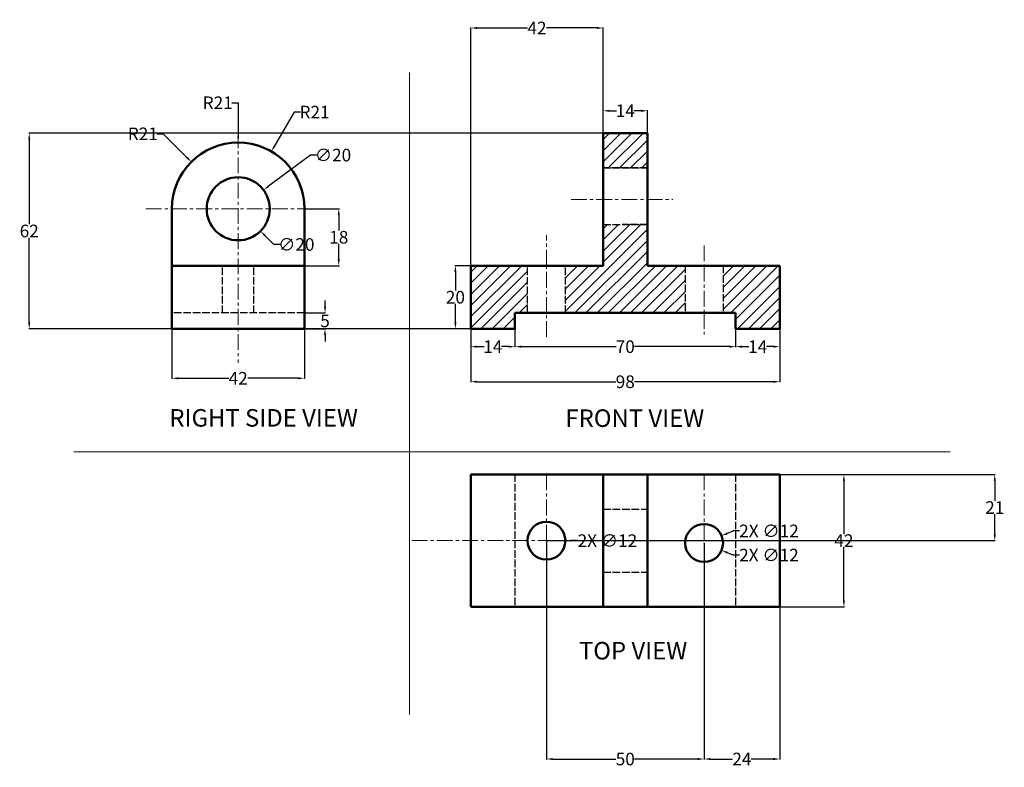
# Model space of a CAD drawing. Units: millimetres. Extents: x -145 to 168, y -286 to 127.
# Tile 1 of 2: x -145 to 168, y -286 to -49. Entities that reach past the tile are written whole.
import ezdxf

# ---------------------------------------------------------------- set-up
doc = ezdxf.new("R2010")
doc.units = ezdxf.units.MM
doc.header["$MEASUREMENT"] = 0
doc.linetypes.add('ACAD_ISO02W100', pattern=[15, 12, -3])
doc.linetypes.add('CENTER', pattern=[2, 1.25, -0.25, 0.25, -0.25])
for name, color, linetype, lineweight in [('M-CNTR', 1, 'CENTER', 18), ('M-CONS', 8, 'Continuous', 18), ('M-DIMS', 2, 'Continuous', 25), ('M-HATC', 8, 'Continuous', 18), ('M-HIDN', 6, 'ACAD_ISO02W100', 25), ('M-OUTL', 7, 'Continuous', 50), ('M-TEXT', 3, 'Continuous', 25)]:
    doc.layers.add(name, color=color, linetype=linetype, lineweight=lineweight)
doc.styles.get("Standard").update_dxf_attribs({"font": 'arial.ttf'})
doc.dimstyles.get("Standard").update_dxf_attribs({"dimtxt": 4, "dimasz": 2, "dimexe": 0.18, "dimexo": 0.0625, "dimgap": 0.09, "dimtad": 0, "dimtih": 1, "dimtoh": 1, "dimdec": 0, "dimzin": 0, "dimdsep": 46, "dimtxsty": 'Standard', "dimcen": 0.09, "dimadec": 0, "dimazin": 0, "dimtfac": 1, "dimtdec": 0, "dimtofl": 0, "dimtmove": 0, "dimatfit": 3, "dimfxl": 1, "dimtolj": 1, "dimtzin": 0, "dimarcsym": 0})

# ---------------------------------------------------------------- blocks, each defined once
blk = doc.blocks.new('*D12')
at = {"layer": 'Defpoints', "color": 0, "transparency": 16777216}
for p in [(40.45, -78.33), (40.45, -85.43), (54.45, -85.43)]:
    blk.add_point(p, dxfattribs=at)
at = {"layer": 'M-DIMS', "color": 0, "lineweight": -2, "transparency": 16777216}
for p, q in [((40.45, -85.37), (40.45, -78.15)), ((42.45, -78.33), (44.69, -78.33)), ((52.45, -78.33), (50.21, -78.33)), ((54.45, -85.37), (54.45, -78.15))]:
    blk.add_line(p, q, dxfattribs=at)
at = {"layer": 'M-DIMS', "color": 0, "transparency": 16777216}
for points in [[(42.45, -78), (42.45, -78.67), (40.45, -78.33)], [(52.45, -78), (52.45, -78.67), (54.45, -78.33)]]:
    blk.add_solid(points, dxfattribs=at)
at = {"layer": 'M-DIMS', "color": 0, "transparency": 16777216, "insert": (47.45, -78.33), "char_height": 4, "attachment_point": 5}
blk.add_mtext('\\A1;14', dxfattribs=at)
blk = doc.blocks.new('*D13')
at = {"layer": 'Defpoints', "color": 0, "transparency": 16777216}
for p in [(-6.42, -127.43), (-1.55, -127.43), (-1.55, -147.43)]:
    blk.add_point(p, dxfattribs=at)
at = {"layer": 'M-DIMS', "color": 0, "lineweight": -2, "transparency": 16777216}
for p, q in [((-1.61, -127.43), (-6.6, -127.43)), ((-6.42, -129.43), (-6.42, -135.3)), ((-6.42, -145.43), (-6.42, -139.56)), ((-1.61, -147.43), (-6.6, -147.43))]:
    blk.add_line(p, q, dxfattribs=at)
at = {"layer": 'M-DIMS', "color": 0, "transparency": 16777216}
for points in [[(-6.75, -129.43), (-6.08, -129.43), (-6.42, -127.43)], [(-6.75, -145.43), (-6.08, -145.43), (-6.42, -147.43)]]:
    blk.add_solid(points, dxfattribs=at)
at = {"layer": 'M-DIMS', "color": 0, "transparency": 16777216, "insert": (-6.42, -137.43), "char_height": 4, "attachment_point": 5}
blk.add_mtext('\\A1;20', dxfattribs=at)
blk = doc.blocks.new('*D14')
at = {"layer": 'Defpoints', "color": 0, "transparency": 16777216}
for p in [(-1.55, -147.43), (12.45, -147.43), (12.45, -153.1)]:
    blk.add_point(p, dxfattribs=at)
at = {"layer": 'M-DIMS', "color": 0, "lineweight": -2, "transparency": 16777216}
for p, q in [((-1.55, -147.49), (-1.55, -153.28)), ((12.45, -147.49), (12.45, -153.28)), ((0.45, -153.1), (2.69, -153.1)), ((10.45, -153.1), (8.21, -153.1))]:
    blk.add_line(p, q, dxfattribs=at)
at = {"layer": 'M-DIMS', "color": 0, "transparency": 16777216}
for points in [[(0.45, -152.77), (0.45, -153.44), (-1.55, -153.1)], [(10.45, -152.77), (10.45, -153.44), (12.45, -153.1)]]:
    blk.add_solid(points, dxfattribs=at)
at = {"layer": 'M-DIMS', "color": 0, "transparency": 16777216, "insert": (5.45, -153.1), "char_height": 4, "attachment_point": 5}
blk.add_mtext('\\A1;14', dxfattribs=at)
blk = doc.blocks.new('*D15')
at = {"layer": 'Defpoints', "color": 0, "transparency": 16777216}
for p in [(12.45, -142.43), (82.45, -142.43), (82.45, -153.1)]:
    blk.add_point(p, dxfattribs=at)
at = {"layer": 'M-DIMS', "color": 0, "lineweight": -2, "transparency": 16777216}
for p, q in [((12.45, -142.49), (12.45, -153.28)), ((82.45, -142.49), (82.45, -153.28)), ((14.45, -153.1), (44.52, -153.1)), ((80.45, -153.1), (50.38, -153.1))]:
    blk.add_line(p, q, dxfattribs=at)
at = {"layer": 'M-DIMS', "color": 0, "transparency": 16777216}
for points in [[(14.45, -152.77), (14.45, -153.44), (12.45, -153.1)], [(80.45, -152.77), (80.45, -153.44), (82.45, -153.1)]]:
    blk.add_solid(points, dxfattribs=at)
at = {"layer": 'M-DIMS', "color": 0, "transparency": 16777216, "insert": (47.45, -153.1), "char_height": 4, "attachment_point": 5}
blk.add_mtext('\\A1;70', dxfattribs=at)
blk = doc.blocks.new('*D16')
at = {"layer": 'Defpoints', "color": 0, "transparency": 16777216}
for p in [(82.45, -147.43), (96.45, -147.43), (96.45, -153.1)]:
    blk.add_point(p, dxfattribs=at)
at = {"layer": 'M-DIMS', "color": 0, "lineweight": -2, "transparency": 16777216}
for p, q in [((82.45, -147.49), (82.45, -153.28)), ((96.45, -147.49), (96.45, -153.28)), ((84.45, -153.1), (86.69, -153.1)), ((94.45, -153.1), (92.21, -153.1))]:
    blk.add_line(p, q, dxfattribs=at)
at = {"layer": 'M-DIMS', "color": 0, "transparency": 16777216}
for points in [[(84.45, -152.77), (84.45, -153.44), (82.45, -153.1)], [(94.45, -152.77), (94.45, -153.44), (96.45, -153.1)]]:
    blk.add_solid(points, dxfattribs=at)
at = {"layer": 'M-DIMS', "color": 0, "transparency": 16777216, "insert": (89.45, -153.1), "char_height": 4, "attachment_point": 5}
blk.add_mtext('\\A1;14', dxfattribs=at)
blk = doc.blocks.new('*D17')
at = {"layer": 'Defpoints', "color": 0, "transparency": 16777216}
for p in [(96.45, -193.6), (116.79, -193.6), (96.45, -235.6)]:
    blk.add_point(p, dxfattribs=at)
at = {"layer": 'M-DIMS', "color": 0, "lineweight": -2, "transparency": 16777216}
for p, q in [((96.51, -193.6), (116.97, -193.6)), ((116.79, -195.6), (116.79, -212.5)), ((116.79, -233.6), (116.79, -216.7)), ((96.51, -235.6), (116.97, -235.6))]:
    blk.add_line(p, q, dxfattribs=at)
at = {"layer": 'M-DIMS', "color": 0, "transparency": 16777216}
for points in [[(116.46, -195.6), (117.13, -195.6), (116.79, -193.6)], [(116.46, -233.6), (117.13, -233.6), (116.79, -235.6)]]:
    blk.add_solid(points, dxfattribs=at)
at = {"layer": 'M-DIMS', "color": 0, "transparency": 16777216, "insert": (116.79, -214.6), "char_height": 4, "attachment_point": 5}
blk.add_mtext('\\A1;42', dxfattribs=at)
blk = doc.blocks.new('*D18')
at = {"layer": 'Defpoints', "color": 0, "transparency": 16777216}
for p in [(-1.55, -147.43), (96.45, -147.43), (96.45, -164.22)]:
    blk.add_point(p, dxfattribs=at)
at = {"layer": 'M-DIMS', "color": 0, "lineweight": -2, "transparency": 16777216}
for p, q in [((-1.55, -147.49), (-1.55, -164.4)), ((96.45, -147.49), (96.45, -164.4)), ((0.45, -164.22), (44.49, -164.22)), ((94.45, -164.22), (50.41, -164.22))]:
    blk.add_line(p, q, dxfattribs=at)
at = {"layer": 'M-DIMS', "color": 0, "transparency": 16777216}
for points in [[(0.45, -163.89), (0.45, -164.56), (-1.55, -164.22)], [(94.45, -163.89), (94.45, -164.56), (96.45, -164.22)]]:
    blk.add_solid(points, dxfattribs=at)
at = {"layer": 'M-DIMS', "color": 0, "transparency": 16777216, "insert": (47.45, -164.22), "char_height": 4, "attachment_point": 5}
blk.add_mtext('\\A1;98', dxfattribs=at)
blk = doc.blocks.new('*D19')
at = {"layer": 'Defpoints', "color": 0, "transparency": 16777216}
for p in [(-96.3, -147.43), (-54.3, -147.43), (-96.3, -163.13)]:
    blk.add_point(p, dxfattribs=at)
at = {"layer": 'M-DIMS', "color": 0, "lineweight": -2, "transparency": 16777216}
for p, q in [((-96.3, -147.49), (-96.3, -163.31)), ((-54.3, -147.49), (-54.3, -163.31)), ((-94.3, -163.13), (-78.31, -163.13)), ((-56.3, -163.13), (-72.28, -163.13))]:
    blk.add_line(p, q, dxfattribs=at)
at = {"layer": 'M-DIMS', "color": 0, "transparency": 16777216}
for points in [[(-94.3, -162.8), (-94.3, -163.46), (-96.3, -163.13)], [(-56.3, -162.8), (-56.3, -163.46), (-54.3, -163.13)]]:
    blk.add_solid(points, dxfattribs=at)
at = {"layer": 'M-DIMS', "color": 0, "transparency": 16777216, "insert": (-75.3, -163.13), "char_height": 4, "attachment_point": 5}
blk.add_mtext('\\A1;42', dxfattribs=at)
blk = doc.blocks.new('*D20')
at = {"layer": 'Defpoints', "color": 0, "transparency": 16777216}
for p in [(-54.3, -142.43), (-47.76, -142.43), (-54.3, -147.43)]:
    blk.add_point(p, dxfattribs=at)
at = {"layer": 'M-DIMS', "color": 0, "lineweight": -2, "transparency": 16777216}
for p, q in [((-47.76, -140.43), (-47.76, -138.43)), ((-54.24, -142.43), (-47.58, -142.43)), ((-54.24, -147.43), (-47.58, -147.43)), ((-47.76, -149.43), (-47.76, -151.43))]:
    blk.add_line(p, q, dxfattribs=at)
at = {"layer": 'M-DIMS', "color": 0, "transparency": 16777216}
for points in [[(-48.09, -140.43), (-47.43, -140.43), (-47.76, -142.43)], [(-48.09, -149.43), (-47.43, -149.43), (-47.76, -147.43)]]:
    blk.add_solid(points, dxfattribs=at)
at = {"layer": 'M-DIMS', "color": 0, "transparency": 16777216, "insert": (-47.76, -144.93), "char_height": 4, "attachment_point": 5}
blk.add_mtext('\\A1;5', dxfattribs=at)
blk = doc.blocks.new('*D21')
at = {"layer": 'Defpoints', "color": 0, "transparency": 16777216}
for p in [(-54.3, -109.39), (-54.3, -127.43), (-43.4, -127.43)]:
    blk.add_point(p, dxfattribs=at)
at = {"layer": 'M-DIMS', "color": 0, "lineweight": -2, "transparency": 16777216}
for p, q in [((-54.24, -109.39), (-43.22, -109.39)), ((-43.4, -111.39), (-43.4, -116.28)), ((-43.4, -125.43), (-43.4, -120.54)), ((-54.24, -127.43), (-43.22, -127.43))]:
    blk.add_line(p, q, dxfattribs=at)
at = {"layer": 'M-DIMS', "color": 0, "transparency": 16777216}
for points in [[(-43.73, -111.39), (-43.07, -111.39), (-43.4, -109.39)], [(-43.73, -125.43), (-43.07, -125.43), (-43.4, -127.43)]]:
    blk.add_solid(points, dxfattribs=at)
at = {"layer": 'M-DIMS', "color": 0, "transparency": 16777216, "insert": (-43.4, -118.41), "char_height": 4, "attachment_point": 5}
blk.add_mtext('\\A1;18', dxfattribs=at)
blk = doc.blocks.new('*D22')
at = {"layer": 'Defpoints', "color": 0, "transparency": 16777216}
for p in [(-64.78, -91.22), (-75.3, -109.39)]:
    blk.add_point(p, dxfattribs=at)
at = {"layer": 'M-DIMS', "color": 0, "lineweight": -2, "transparency": 16777216}
for p, q in [((-57.56, -78.75), (-63.78, -89.49)), ((-55.56, -78.75), (-57.56, -78.75)), ((-75.39, -109.39), (-75.21, -109.39)), ((-75.3, -109.48), (-75.3, -109.3))]:
    blk.add_line(p, q, dxfattribs=at)
at = {"layer": 'M-DIMS', "color": 0, "transparency": 16777216}
blk.add_solid([(-64.06, -89.32), (-63.49, -89.65), (-64.78, -91.22)], dxfattribs=at)
at = {"layer": 'M-DIMS', "color": 0, "transparency": 16777216, "insert": (-51.08, -78.75), "char_height": 4, "attachment_point": 5}
blk.add_mtext('\\A1;R21', dxfattribs=at)
blk = doc.blocks.new('*D23')
at = {"layer": 'Defpoints', "color": 0, "transparency": 16777216}
for p in [(-67.27, -103.43), (-83.33, -115.35)]:
    blk.add_point(p, dxfattribs=at)
at = {"layer": 'M-DIMS', "color": 0, "lineweight": -2, "transparency": 16777216}
for p, q in [((-52.35, -92.37), (-65.66, -102.24)), ((-50.35, -92.37), (-52.35, -92.37)), ((-75.39, -109.39), (-75.21, -109.39)), ((-75.3, -109.48), (-75.3, -109.3))]:
    blk.add_line(p, q, dxfattribs=at)
at = {"layer": 'M-DIMS', "color": 0, "transparency": 16777216}
blk.add_solid([(-65.86, -101.98), (-65.46, -102.51), (-67.27, -103.43)], dxfattribs=at)
at = {"layer": 'M-DIMS', "color": 0, "transparency": 16777216, "insert": (-45.23, -92.37), "char_height": 4, "attachment_point": 5}
blk.add_mtext('\\A1;∅20', dxfattribs=at)
blk = doc.blocks.new('*D24')
at = {"layer": 'Defpoints', "color": 0, "transparency": 16777216}
for p in [(22.45, -214.6), (72.45, -215.35), (72.45, -283.82)]:
    blk.add_point(p, dxfattribs=at)
at = {"layer": 'M-DIMS', "color": 0, "lineweight": -2, "transparency": 16777216}
for p, q in [((22.45, -214.66), (22.45, -284)), ((72.45, -215.41), (72.45, -284)), ((24.45, -283.82), (44.5, -283.82)), ((70.45, -283.82), (50.4, -283.82))]:
    blk.add_line(p, q, dxfattribs=at)
at = {"layer": 'M-DIMS', "color": 0, "transparency": 16777216}
for points in [[(24.45, -283.49), (24.45, -284.16), (22.45, -283.82)], [(70.45, -283.49), (70.45, -284.16), (72.45, -283.82)]]:
    blk.add_solid(points, dxfattribs=at)
at = {"layer": 'M-DIMS', "color": 0, "transparency": 16777216, "insert": (47.45, -283.82), "char_height": 4, "attachment_point": 5}
blk.add_mtext('\\A1;50', dxfattribs=at)
blk = doc.blocks.new('*D25')
at = {"layer": 'Defpoints', "color": 0, "transparency": 16777216}
for p in [(72.45, -215.35), (96.45, -235.6), (96.45, -283.82)]:
    blk.add_point(p, dxfattribs=at)
at = {"layer": 'M-DIMS', "color": 0, "lineweight": -2, "transparency": 16777216}
for p, q in [((72.45, -215.41), (72.45, -284)), ((96.45, -235.66), (96.45, -284)), ((74.45, -283.82), (81.47, -283.82)), ((94.45, -283.82), (87.43, -283.82))]:
    blk.add_line(p, q, dxfattribs=at)
at = {"layer": 'M-DIMS', "color": 0, "transparency": 16777216}
for points in [[(74.45, -283.49), (74.45, -284.16), (72.45, -283.82)], [(94.45, -283.49), (94.45, -284.16), (96.45, -283.82)]]:
    blk.add_solid(points, dxfattribs=at)
at = {"layer": 'M-DIMS', "color": 0, "transparency": 16777216, "insert": (84.45, -283.82), "char_height": 4, "attachment_point": 5}
blk.add_mtext('\\A1;24', dxfattribs=at)
blk = doc.blocks.new('*D26')
at = {"layer": 'Defpoints', "color": 0, "transparency": 16777216}
for p in [(96.45, -193.6), (164.63, -193.6), (22.45, -214.6)]:
    blk.add_point(p, dxfattribs=at)
at = {"layer": 'M-DIMS', "color": 0, "lineweight": -2, "transparency": 16777216}
for p, q in [((96.51, -193.6), (164.81, -193.6)), ((164.63, -195.6), (164.63, -202)), ((164.63, -212.6), (164.63, -206.2)), ((22.51, -214.6), (164.81, -214.6))]:
    blk.add_line(p, q, dxfattribs=at)
at = {"layer": 'M-DIMS', "color": 0, "transparency": 16777216}
for points in [[(164.3, -195.6), (164.96, -195.6), (164.63, -193.6)], [(164.3, -212.6), (164.96, -212.6), (164.63, -214.6)]]:
    blk.add_solid(points, dxfattribs=at)
at = {"layer": 'M-DIMS', "color": 0, "transparency": 16777216, "insert": (164.63, -204.1), "char_height": 4, "attachment_point": 5}
blk.add_mtext('\\A1;21', dxfattribs=at)
blk = doc.blocks.new('*D27')
at = {"layer": 'Defpoints', "color": 0, "transparency": 16777216}
for p in [(40.45, -85.43), (-141.57, -147.43), (-1.55, -147.43)]:
    blk.add_point(p, dxfattribs=at)
at = {"layer": 'M-DIMS', "color": 0, "lineweight": -2, "transparency": 16777216}
for p, q in [((40.39, -85.43), (-141.75, -85.43)), ((-141.57, -87.43), (-141.57, -114.3)), ((-141.57, -145.43), (-141.57, -118.56)), ((-1.61, -147.43), (-141.75, -147.43))]:
    blk.add_line(p, q, dxfattribs=at)
at = {"layer": 'M-DIMS', "color": 0, "transparency": 16777216}
for points in [[(-141.9, -87.43), (-141.24, -87.43), (-141.57, -85.43)], [(-141.9, -145.43), (-141.24, -145.43), (-141.57, -147.43)]]:
    blk.add_solid(points, dxfattribs=at)
at = {"layer": 'M-DIMS', "color": 0, "transparency": 16777216, "insert": (-141.57, -116.43), "char_height": 4, "attachment_point": 5}
blk.add_mtext('\\A1;62', dxfattribs=at)
blk = doc.blocks.new('*D28')
at = {"layer": 'Defpoints', "color": 0, "transparency": 16777216}
for p in [(-90.15, -94.55), (-75.3, -109.39)]:
    blk.add_point(p, dxfattribs=at)
at = {"layer": 'M-DIMS', "color": 0, "lineweight": -2, "transparency": 16777216}
for p, q in [((-101.07, -85.64), (-99.07, -85.64)), ((-99.07, -85.64), (-91.57, -93.13)), ((-75.39, -109.39), (-75.21, -109.39)), ((-75.3, -109.48), (-75.3, -109.3))]:
    blk.add_line(p, q, dxfattribs=at)
at = {"layer": 'M-DIMS', "color": 0, "transparency": 16777216}
blk.add_solid([(-91.33, -92.9), (-91.8, -93.37), (-90.15, -94.55)], dxfattribs=at)
at = {"layer": 'M-DIMS', "color": 0, "transparency": 16777216, "insert": (-105.55, -85.64), "char_height": 4, "attachment_point": 5}
blk.add_mtext('\\A1;R21', dxfattribs=at)
blk = doc.blocks.new('*D29')
at = {"layer": 'Defpoints', "color": 0, "transparency": 16777216}
for p in [(-82.37, -102.32), (-68.23, -116.47)]:
    blk.add_point(p, dxfattribs=at)
at = {"layer": 'M-DIMS', "color": 0, "lineweight": -2, "transparency": 16777216}
for p, q in [((-75.39, -109.39), (-75.21, -109.39)), ((-75.3, -109.48), (-75.3, -109.3)), ((-63.99, -120.71), (-66.82, -117.88)), ((-61.99, -120.71), (-63.99, -120.71))]:
    blk.add_line(p, q, dxfattribs=at)
at = {"layer": 'M-DIMS', "color": 0, "transparency": 16777216}
blk.add_solid([(-66.58, -117.65), (-67.05, -118.12), (-68.23, -116.47)], dxfattribs=at)
at = {"layer": 'M-DIMS', "color": 0, "transparency": 16777216, "insert": (-56.87, -120.71), "char_height": 4, "attachment_point": 5}
blk.add_mtext('\\A1;∅20', dxfattribs=at)
blk = doc.blocks.new('*D30')
at = {"layer": 'Defpoints', "color": 0, "transparency": 16777216}
for p in [(16.45, -214.6), (28.45, -214.6)]:
    blk.add_point(p, dxfattribs=at)
at = {"layer": 'M-DIMS', "color": 0, "lineweight": -2, "transparency": 16777216}
for p, q in [((22.36, -214.6), (22.54, -214.6)), ((22.45, -214.69), (22.45, -214.51)), ((32.45, -214.6), (30.45, -214.6))]:
    blk.add_line(p, q, dxfattribs=at)
at = {"layer": 'M-DIMS', "color": 0, "transparency": 16777216}
blk.add_solid([(30.45, -214.27), (30.45, -214.93), (28.45, -214.6)], dxfattribs=at)
at = {"layer": 'M-DIMS', "color": 0, "transparency": 16777216, "insert": (41.79, -214.6), "char_height": 4, "attachment_point": 5}
blk.add_mtext('\\A1;2X ∅12', dxfattribs=at)
blk = doc.blocks.new('*D31')
at = {"layer": 'Defpoints', "color": 0, "transparency": 16777216}
for p in [(66.91, -213.05), (77.99, -217.65)]:
    blk.add_point(p, dxfattribs=at)
at = {"layer": 'M-DIMS', "color": 0, "lineweight": -2, "transparency": 16777216}
for p, q in [((72.36, -215.35), (72.54, -215.35)), ((72.45, -215.44), (72.45, -215.26)), ((81.69, -219.18), (79.84, -218.41)), ((83.69, -219.18), (81.69, -219.18))]:
    blk.add_line(p, q, dxfattribs=at)
at = {"layer": 'M-DIMS', "color": 0, "transparency": 16777216}
blk.add_solid([(79.97, -218.11), (79.71, -218.72), (77.99, -217.65)], dxfattribs=at)
at = {"layer": 'M-DIMS', "color": 0, "transparency": 16777216, "insert": (93.02, -219.18), "char_height": 4, "attachment_point": 5}
blk.add_mtext('\\A1;2X ∅12', dxfattribs=at)
blk = doc.blocks.new('*D32')
at = {"layer": 'Defpoints', "color": 0, "transparency": 16777216}
for p in [(40.45, -52.08), (-1.55, -127.43), (40.45, -127.43)]:
    blk.add_point(p, dxfattribs=at)
at = {"layer": 'M-DIMS', "color": 0, "lineweight": -2, "transparency": 16777216}
for p, q in [((-1.55, -127.37), (-1.55, -51.9)), ((0.45, -52.08), (16.44, -52.08)), ((38.45, -52.08), (22.47, -52.08)), ((40.45, -127.37), (40.45, -51.9))]:
    blk.add_line(p, q, dxfattribs=at)
at = {"layer": 'M-DIMS', "color": 0, "transparency": 16777216}
for points in [[(0.45, -51.74), (0.45, -52.41), (-1.55, -52.08)], [(38.45, -51.74), (38.45, -52.41), (40.45, -52.08)]]:
    blk.add_solid(points, dxfattribs=at)
at = {"layer": 'M-DIMS', "color": 0, "transparency": 16777216, "insert": (19.45, -52.08), "char_height": 4, "attachment_point": 5}
blk.add_mtext('\\A1;42', dxfattribs=at)
blk = doc.blocks.new('*D33')
at = {"layer": 'Defpoints', "color": 0, "transparency": 16777216}
for p in [(-75.3, -88.39), (-75.3, -109.39)]:
    blk.add_point(p, dxfattribs=at)
at = {"layer": 'M-DIMS', "color": 0, "lineweight": -2, "transparency": 16777216}
for p, q in [((-77.3, -75.79), (-75.3, -75.79)), ((-75.3, -75.79), (-75.3, -86.39)), ((-75.39, -109.39), (-75.21, -109.39)), ((-75.3, -109.48), (-75.3, -109.3))]:
    blk.add_line(p, q, dxfattribs=at)
at = {"layer": 'M-DIMS', "color": 0, "transparency": 16777216}
blk.add_solid([(-74.97, -86.39), (-75.63, -86.39), (-75.3, -88.39)], dxfattribs=at)
at = {"layer": 'M-DIMS', "color": 0, "transparency": 16777216, "insert": (-81.78, -75.79), "char_height": 4, "attachment_point": 5}
blk.add_mtext('\\A1;R21', dxfattribs=at)
blk = doc.blocks.new('*D34')
at = {"layer": 'Defpoints', "color": 0, "transparency": 16777216}
for p in [(77.99, -213.05), (66.91, -217.65)]:
    blk.add_point(p, dxfattribs=at)
at = {"layer": 'M-DIMS', "color": 0, "lineweight": -2, "transparency": 16777216}
for p, q in [((81.69, -211.52), (79.84, -212.28)), ((83.69, -211.52), (81.69, -211.52)), ((72.36, -215.35), (72.54, -215.35)), ((72.45, -215.44), (72.45, -215.26))]:
    blk.add_line(p, q, dxfattribs=at)
at = {"layer": 'M-DIMS', "color": 0, "transparency": 16777216}
blk.add_solid([(79.71, -211.98), (79.97, -212.59), (77.99, -213.05)], dxfattribs=at)
at = {"layer": 'M-DIMS', "color": 0, "transparency": 16777216, "insert": (93.03, -211.52), "char_height": 4, "attachment_point": 5}
blk.add_mtext('\\A1;2X ∅12', dxfattribs=at)

msp = doc.modelspace()

# ---------------------------------------------------------------- hatches: boundary and pattern name
at = {"layer": 'M-HATC'}
h = msp.add_hatch(dxfattribs=at)
h.set_pattern_fill('ANSI31', color=256, scale=20)
h.set_pattern_definition([(45, (-165.473, 95.536), (-1.767767, 1.767767), [])])
h.paths.add_polyline_path([(96.45, -127.43), (78.45, -127.43), (78.45, -142.43), (82.45, -142.43), (82.45, -147.43), (96.45, -147.43)])
h.paths.add_polyline_path([(66.45, -127.43), (54.45, -127.43), (54.45, -114.39), (40.45, -114.39), (40.45, -127.43), (28.45, -127.43), (28.45, -142.43), (66.45, -142.43)])
h.paths.add_polyline_path([(16.45, -127.43), (-1.55, -127.43), (-1.55, -147.43), (12.45, -147.43), (12.45, -142.43), (16.45, -142.43)])
h.paths.add_polyline_path([(54.45, -85.43), (40.45, -85.43), (40.45, -96.43), (54.45, -96.43)])

# ---------------------------------------------------------------- linework, layer by layer
at = {"layer": 'M-CNTR', "ltscale": 4}
for p, q in [((-75.3, -77.15), (-75.3, -158.19)), ((30.25, -106.43), (62.56, -106.43)), ((-104.6, -109.39), (-43.99, -109.39)), ((22.45, -193.6), (22.45, -235.6)), ((72.45, -193.6), (72.45, -235.6)), ((-20.27, -214.6), (107.77, -214.6))]:
    msp.add_line(p, q, dxfattribs=at)
for points in [[(22.45, -150.02), (22.45, -142.43), (22.45, -127.43), (22.45, -117.74)], [(72.45, -121.03), (72.45, -127.43), (72.45, -142.43), (72.45, -149.23)]]:
    msp.add_lwpolyline(points, dxfattribs=at)
at = {"layer": 'M-CONS'}
for p, q in [((-20.95, -66.23), (-20.95, -269.67)), ((-127.42, -186.48), (150.48, -186.48))]:
    msp.add_line(p, q, dxfattribs=at)
at = {"layer": 'M-HIDN', "ltscale": 0.2}
for p, q in [((54.45, -96.43), (40.45, -96.43)), ((40.45, -96.43), (54.45, -96.43)), ((40.45, -114.39), (54.45, -114.39)), ((54.45, -114.39), (46.5, -114.39)), ((-80.3, -142.43), (-80.3, -127.43)), ((-70.3, -142.43), (-70.3, -127.43)), ((16.45, -142.43), (16.45, -127.43)), ((28.45, -142.43), (28.45, -127.43)), ((66.45, -127.43), (66.45, -142.43)), ((78.45, -127.43), (78.45, -142.43)), ((-54.3, -142.43), (-96.3, -142.43)), ((12.45, -193.6), (12.45, -235.6)), ((82.45, -193.6), (82.45, -235.6)), ((40.45, -204.6), (54.45, -204.6)), ((40.45, -224.6), (54.45, -224.6))]:
    msp.add_line(p, q, dxfattribs=at)
at = {"layer": 'M-OUTL'}
for p, q in [((54.45, -85.43), (40.45, -85.43)), ((40.45, -85.43), (40.45, -106.43)), ((54.45, -106.43), (54.45, -85.43)), ((40.45, -106.43), (40.45, -127.43)), ((54.45, -127.43), (54.45, -106.43)), ((-96.3, -130.39), (-96.3, -109.39)), ((-54.3, -109.39), (-54.3, -127.43)), ((-96.3, -147.43), (-96.3, -127.43)), ((-96.3, -127.43), (-54.3, -127.43)), ((-54.3, -127.43), (-54.3, -147.43)), ((-1.55, -147.43), (-1.55, -127.43)), ((40.45, -127.43), (-1.55, -127.43)), ((96.45, -127.43), (54.45, -127.43)), ((96.45, -147.43), (96.45, -127.43)), ((12.45, -147.43), (12.45, -142.43)), ((12.45, -142.43), (82.45, -142.43)), ((82.45, -142.43), (82.45, -147.43)), ((-54.3, -147.43), (-96.3, -147.43)), ((-1.55, -147.43), (12.45, -147.43)), ((82.45, -147.43), (96.45, -147.43)), ((-1.55, -193.6), (-1.55, -235.6)), ((96.45, -193.6), (-1.55, -193.6)), ((40.45, -193.6), (40.45, -235.6)), ((54.45, -193.6), (54.45, -235.6)), ((96.45, -235.6), (96.45, -193.6)), ((-1.55, -235.6), (96.45, -235.6))]:
    msp.add_line(p, q, dxfattribs=at)
for centre, radius in [((-75.3, -109.39), 10), ((22.45, -214.6), 6), ((72.45, -215.35), 6)]:
    msp.add_circle(centre, radius, dxfattribs=at)
msp.add_arc((-75.3, -109.39), 21, 0, 180, dxfattribs=at)

# ---------------------------------------------------------------- texts
at = {"layer": 'M-TEXT'}
for s, p in [('RIGHT SIDE VIEW', (-97.14, -178.45)), ('FRONT VIEW', (28.47, -178.54)), ('TOP VIEW', (32.76, -252.26))]:
    msp.add_text(s, height=5.554, dxfattribs=at).set_placement(p)

# ---------------------------------------------------------------- dimensions: what is measured, and where the dimension line sits
at = {"layer": 'M-DIMS'}
for base, p1, p2, override, picture, middle in [((40.45, -52.08), (-1.55, -127.43), (40.45, -127.43), {"dimdec": 0, "dimlfac": 1, "dimrnd": 0, "dimzin": 0, "dimdsep": 46, "dimlunit": 2}, '*D32', (19.45, -52.08)), ((40.45, -78.33), (54.45, -85.43), (40.45, -85.43), {"dimclrd": 0, "dimclre": 0, "dimclrt": 0}, '*D12', (47.45, -78.33)), ((82.45, -153.1), (12.45, -142.43), (82.45, -142.43), {"dimclrd": 0, "dimclre": 0, "dimclrt": 0}, '*D15', (47.45, -153.1)), ((-96.3, -163.13), (-54.3, -147.43), (-96.3, -147.43), {"dimclrd": 0, "dimclre": 0, "dimclrt": 0}, '*D19', (-75.3, -163.13)), ((12.45, -153.1), (-1.55, -147.43), (12.45, -147.43), {"dimclrd": 0, "dimclre": 0, "dimclrt": 0}, '*D14', (5.45, -153.1)), ((96.45, -164.22), (-1.55, -147.43), (96.45, -147.43), {"dimclrd": 0, "dimclre": 0, "dimclrt": 0}, '*D18', (47.45, -164.22)), ((96.45, -153.1), (82.45, -147.43), (96.45, -147.43), {"dimclrd": 0, "dimclre": 0, "dimclrt": 0}, '*D16', (89.45, -153.1)), ((72.45, -283.82), (22.45, -214.6), (72.45, -215.35), {"dimdec": 0, "dimlfac": 1, "dimrnd": 0, "dimzin": 0, "dimdsep": 46, "dimlunit": 2}, '*D24', (47.45, -283.82)), ((96.45, -283.82), (72.45, -215.35), (96.45, -235.6), {"dimdec": 0, "dimlfac": 1, "dimrnd": 0, "dimzin": 0, "dimdsep": 46, "dimlunit": 2}, '*D25', (84.45, -283.82))]:
    dim = msp.add_linear_dim(base=base, p1=p1, p2=p2, dimstyle='Standard', override=override, dxfattribs=at)
    dim.commit()
    dim.dimension.update_dxf_attribs({"geometry": picture, "text_midpoint": middle})
for mpoint, override, picture, middle in [((-75.3, -88.39), {"dimdec": 0, "dimlfac": 1, "dimrnd": 0, "dimzin": 0, "dimdsep": 46, "dimlunit": 2}, '*D33', (-81.78, -75.79)), ((-64.78, -91.22), {"dimclrd": 0, "dimclre": 0, "dimclrt": 0}, '*D22', (-51.08, -78.75)), ((-90.15, -94.55), {"dimdec": 0, "dimlfac": 1, "dimrnd": 0, "dimzin": 0, "dimdsep": 46, "dimlunit": 2}, '*D28', (-105.55, -85.64))]:
    dim = msp.add_radius_dim(center=(-75.3, -109.39), mpoint=mpoint, dimstyle='Standard', override=override, dxfattribs=at)
    dim.commit()
    dim.dimension.update_dxf_attribs({"geometry": picture, "text_midpoint": middle, "dimtype": 164})
for base, p1, p2, override, picture, middle in [((-141.57, -147.43), (40.45, -85.43), (-1.55, -147.43), {"dimdec": 0, "dimlfac": 1, "dimrnd": 0, "dimzin": 0, "dimdsep": 46, "dimlunit": 2}, '*D27', (-141.57, -116.43)), ((-43.4, -127.43), (-54.3, -109.39), (-54.3, -127.43), {"dimclrd": 0, "dimclre": 0, "dimclrt": 0}, '*D21', (-43.4, -118.41)), ((-6.42, -127.43), (-1.55, -147.43), (-1.55, -127.43), {"dimclrd": 0, "dimclre": 0, "dimclrt": 0}, '*D13', (-6.42, -137.43)), ((-47.76, -142.43), (-54.3, -147.43), (-54.3, -142.43), {"dimclrd": 0, "dimclre": 0, "dimclrt": 0}, '*D20', (-47.76, -144.93)), ((164.63, -193.6), (22.45, -214.6), (96.45, -193.6), {"dimdec": 0, "dimlfac": 1, "dimrnd": 0, "dimzin": 0, "dimdsep": 46, "dimlunit": 2}, '*D26', (164.63, -204.1)), ((116.79, -193.6), (96.45, -235.6), (96.45, -193.6), {"dimclrd": 0, "dimclre": 0, "dimclrt": 0}, '*D17', (116.79, -214.6))]:
    dim = msp.add_linear_dim(base=base, p1=p1, p2=p2, angle=90, dimstyle='Standard', override=override, dxfattribs=at)
    dim.commit()
    dim.dimension.update_dxf_attribs({"geometry": picture, "text_midpoint": middle})
for p1, p2, override, picture, middle in [((-83.33, -115.35), (-67.27, -103.43), {"dimclrd": 0, "dimclre": 0, "dimclrt": 0}, '*D23', (-45.23, -92.37)), ((-82.37, -102.32), (-68.23, -116.47), {"dimdec": 0, "dimlfac": 1, "dimrnd": 0, "dimzin": 0, "dimdsep": 46, "dimlunit": 2}, '*D29', (-56.87, -120.71))]:
    dim = msp.add_diameter_dim_2p(p1=p1, p2=p2, dimstyle='Standard', override=override, dxfattribs=at)
    dim.commit()
    dim.dimension.update_dxf_attribs({"geometry": picture, "text_midpoint": middle, "dimtype": 163})
for p1, p2, picture, middle in [((66.91, -217.65), (77.99, -213.05), '*D34', (93.03, -211.52)), ((16.45, -214.6), (28.45, -214.6), '*D30', (32.45, -214.6)), ((66.91, -213.05), (77.99, -217.65), '*D31', (93.02, -219.18))]:
    dim = msp.add_diameter_dim_2p(p1=p1, p2=p2, text='2X <>', dimstyle='Standard', override={"dimdec": 0, "dimlfac": 1, "dimrnd": 0, "dimzin": 0, "dimdsep": 46, "dimlunit": 2}, dxfattribs=at)
    dim.commit()
    dim.dimension.update_dxf_attribs({"geometry": picture, "text_midpoint": middle, "dimtype": 163})

doc.saveas('drawing.dxf')
